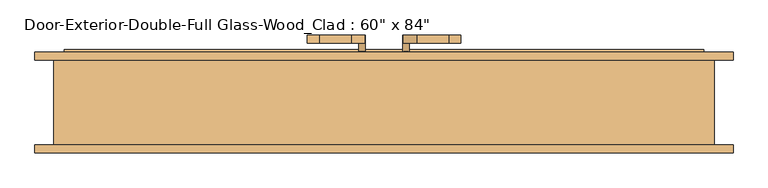
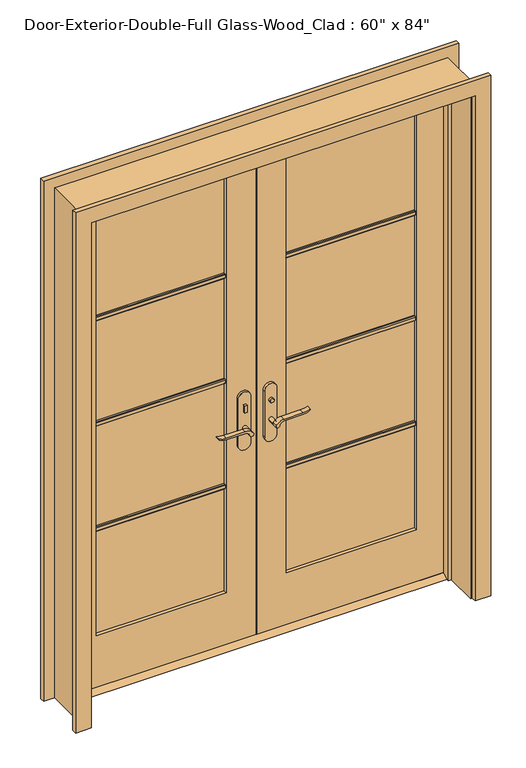
"""IFC4 building model written with IfcOpenShell, lengths in millimetres: door geometry."""

from ifc_helpers import new_model, si_unit, point, frame, frame_2d, origin, place, context, project, spatial, polyline, circle_curve, trimmed, segment, composite_curve, outline, extrude, faceted_brep, source, transform, mapped, element, save


def door_34824ff4(model_context):
    return source(origin(), model_context, "Body", "SolidModel", [
        extrude(outline(polyline([(63.5, 12.7), (98.425, 12.7), (123.825, 0.0), (38.1, 0.0), (63.5, 12.7)])), frame((-762.0, 0.0, 0.0), z_axis=(1.0, 0.0, 0.0), x_axis=(0.0, 1.0, 0.0)), (0.0, 0.0, 1.0), 1524.0),
        extrude(outline(polyline([(-47.4019111, 43.5), (-57.4019111, 43.5), (-57.4019111, 53.5), (-47.4019111, 53.5), (-47.4019111, 43.5)])), frame((0.0, 0.0, 981.9), z_axis=(0.0, 0.0, 1.0), x_axis=(1.0, 0.0, 0.0)), (0.0, 0.0, 1.0), 30.0),
        extrude(outline(composite_curve([segment(trimmed(circle_curve(frame_2d((996.9, -52.4019111)), 8.0), [point((996.9, -60.4019111))], [point((996.9, -44.4019111))], False, "CARTESIAN"), True, "CONTINUOUS"), segment(trimmed(circle_curve(frame_2d((996.9, -52.4019111)), 8.0), [point((996.9, -44.4019111))], [point((996.9, -60.4019111))], False, "CARTESIAN"), True, "CONTINUOUS")], self_intersect=False)), frame((0.0, 108.425, 0.0), z_axis=(0.0, 1.0, 0.0), x_axis=(0.0, 0.0, 1.0)), (0.0, 0.0, 1.0), 10.0),
        extrude(outline(composite_curve([segment(trimmed(circle_curve(frame_2d((897.1555521, -76.0694241)), 37.2832219), [point((919.0523287, -45.8937749))], [point((934.4, -77.7693445))], False, "CARTESIAN"), True, "CONTINUOUS"), segment(polyline([(934.4, -77.7693445), (934.4, -154.045502)]), True, "CONTINUOUS"), segment(trimmed(circle_curve(frame_2d((1017.6850638, -153.9791202)), 83.2850902), [point((934.4, -154.045502))], [point((939.4, -182.4019111))], True, "CARTESIAN"), True, "CONTINUOUS"), segment(polyline([(939.4, -182.4019111), (936.6135558, -182.4019111)]), True, "CONTINUOUS"), segment(trimmed(circle_curve(frame_2d((986.6709207, -150.4622499)), 59.3791355), [point((936.6135558, -182.4019111))], [point((927.4, -154.045502))], False, "CARTESIAN"), True, "CONTINUOUS"), segment(polyline([(927.4, -154.045502), (927.4, -77.7881013)]), True, "CONTINUOUS"), segment(trimmed(circle_curve(frame_2d((909.2738613, -77.7881013)), 18.1261387), [point((927.4, -77.7881013))], [point((914.4, -60.4019111))], True, "CARTESIAN"), True, "CONTINUOUS"), segment(trimmed(circle_curve(frame_2d((914.4, -52.4019111)), 8.0), [point((914.4, -60.4019111))], [point((919.0523287, -45.8937749))], False, "CARTESIAN"), True, "CONTINUOUS")], self_intersect=False)), frame((0.0, 3.5, 0.0), z_axis=(0.0, 1.0, 0.0), x_axis=(0.0, 0.0, 1.0)), (0.0, 0.0, 1.0), 20.0),
        extrude(outline(composite_curve([segment(trimmed(circle_curve(frame_2d((914.4, -52.4019111)), 8.0), [point((914.3999903, -60.4019111))], [point((919.0523287, -45.8937749))], False, "CARTESIAN"), True, "CONTINUOUS"), segment(trimmed(circle_curve(frame_2d((897.1555521, -76.0694241)), 37.2832219), [point((919.0523287, -45.8937749))], [point((934.4, -77.7693445))], False, "CARTESIAN"), True, "CONTINUOUS"), segment(polyline([(934.4, -77.7693445), (934.4, -154.045502)]), True, "CONTINUOUS"), segment(trimmed(circle_curve(frame_2d((1017.6850638, -153.9791202)), 83.2850902), [point((934.4, -154.045502))], [point((939.4, -182.4019111))], True, "CARTESIAN"), True, "CONTINUOUS"), segment(polyline([(939.4, -182.4019111), (936.6135558, -182.4019111)]), True, "CONTINUOUS"), segment(trimmed(circle_curve(frame_2d((986.6709207, -150.4622499)), 59.3791355), [point((936.6135558, -182.4019111))], [point((927.4, -154.045502))], False, "CARTESIAN"), True, "CONTINUOUS"), segment(polyline([(927.4, -154.045502), (927.4, -77.788099)]), True, "CONTINUOUS"), segment(trimmed(circle_curve(frame_2d((909.2738682, -77.788099)), 18.1261318), [point((927.4, -77.788099))], [point((914.3999903, -60.4019111))], True, "CARTESIAN"), True, "CONTINUOUS")], self_intersect=False)), frame((0.0, 138.425, 0.0), z_axis=(0.0, 1.0, 0.0), x_axis=(0.0, 0.0, 1.0)), (0.0, 0.0, 1.0), 20.0),
        extrude(outline(composite_curve([segment(trimmed(circle_curve(frame_2d((914.4, -52.4019111)), 8.0), [point((914.4, -60.4019111))], [point((914.4, -44.4019111))], False, "CARTESIAN"), True, "CONTINUOUS"), segment(trimmed(circle_curve(frame_2d((914.4, -52.4019111)), 8.0), [point((914.4, -44.4019111))], [point((914.4, -60.4019111))], False, "CARTESIAN"), True, "CONTINUOUS")], self_intersect=False)), frame((0.0, 23.5, 0.0), z_axis=(0.0, 1.0, 0.0), x_axis=(0.0, 0.0, 1.0)), (0.0, 0.0, 1.0), 30.0),
        extrude(outline(composite_curve([segment(trimmed(circle_curve(frame_2d((914.4, -52.4019111)), 8.0), [point((914.4, -60.4019111))], [point((914.4, -44.4019111))], False, "CARTESIAN"), True, "CONTINUOUS"), segment(trimmed(circle_curve(frame_2d((914.4, -52.4019111)), 8.0), [point((914.4, -44.4019111))], [point((914.4, -60.4019111))], False, "CARTESIAN"), True, "CONTINUOUS")], self_intersect=False)), frame((0.0, 108.425, 0.0), z_axis=(0.0, 1.0, 0.0), x_axis=(0.0, 0.0, 1.0)), (0.0, 0.0, 1.0), 30.0),
        extrude(outline(composite_curve([segment(polyline([(844.4, -27.4019111), (1039.4, -27.4019111)]), True, "CONTINUOUS"), segment(trimmed(circle_curve(frame_2d((1039.4, -52.4019111)), 25.0), [point((1039.4, -27.4019111))], [point((1039.4, -77.4019111))], False, "CARTESIAN"), True, "CONTINUOUS"), segment(polyline([(1039.4, -77.4019111), (844.4, -77.4019111)]), True, "CONTINUOUS"), segment(trimmed(circle_curve(frame_2d((844.4, -52.4019111)), 25.0), [point((844.4, -77.4019111))], [point((844.4, -27.4019111))], False, "CARTESIAN"), True, "CONTINUOUS")], self_intersect=False)), frame((0.0, 53.5, 0.0), z_axis=(0.0, 1.0, 0.0), x_axis=(0.0, 0.0, 1.0)), (0.0, 0.0, 1.0), 10.0),
        extrude(outline(composite_curve([segment(polyline([(844.4, -27.4019111), (1039.4, -27.4019111)]), True, "CONTINUOUS"), segment(trimmed(circle_curve(frame_2d((1039.4, -52.4019111)), 25.0), [point((1039.4, -27.4019111))], [point((1039.4, -77.4019111))], False, "CARTESIAN"), True, "CONTINUOUS"), segment(polyline([(1039.4, -77.4019111), (844.4, -77.4019111)]), True, "CONTINUOUS"), segment(trimmed(circle_curve(frame_2d((844.4, -52.4019111)), 25.0), [point((844.4, -77.4019111))], [point((844.4, -27.4019111))], False, "CARTESIAN"), True, "CONTINUOUS")], self_intersect=False)), frame((0.0, 98.425, 0.0), z_axis=(0.0, 1.0, 0.0), x_axis=(0.0, 0.0, 1.0)), (0.0, 0.0, 1.0), 10.0),
        extrude(outline(polyline([(47.3875, 118.425), (57.3875, 118.425), (57.3875, 108.425), (47.3875, 108.425), (47.3875, 118.425)])), frame((0.0, 0.0, 981.9), z_axis=(0.0, 0.0, 1.0), x_axis=(1.0, 0.0, 0.0)), (0.0, 0.0, 1.0), 30.0),
        extrude(outline(composite_curve([segment(trimmed(circle_curve(frame_2d((996.9, 52.3875)), 8.0), [point((996.9, 60.3875))], [point((996.9, 44.3875))], False, "CARTESIAN"), True, "CONTINUOUS"), segment(trimmed(circle_curve(frame_2d((996.9, 52.3875)), 8.0), [point((996.9, 44.3875))], [point((996.9, 60.3875))], False, "CARTESIAN"), True, "CONTINUOUS")], self_intersect=False)), frame((0.0, 43.5, 0.0), z_axis=(0.0, 1.0, 0.0), x_axis=(0.0, 0.0, 1.0)), (0.0, 0.0, 1.0), 10.0),
        extrude(outline(composite_curve([segment(trimmed(circle_curve(frame_2d((914.4, 52.3875)), 8.0), [point((919.0523287, 45.8793637))], [point((914.4, 60.3875))], False, "CARTESIAN"), True, "CONTINUOUS"), segment(trimmed(circle_curve(frame_2d((909.2738613, 77.7736901)), 18.1261387), [point((914.4, 60.3875))], [point((927.4, 77.7736901))], True, "CARTESIAN"), True, "CONTINUOUS"), segment(polyline([(927.4, 77.7736901), (927.4, 154.0310909)]), True, "CONTINUOUS"), segment(trimmed(circle_curve(frame_2d((986.6709207, 150.4478388)), 59.3791355), [point((927.4, 154.0310909))], [point((936.6135558, 182.3875))], False, "CARTESIAN"), True, "CONTINUOUS"), segment(polyline([(936.6135558, 182.3875), (939.4, 182.3875)]), True, "CONTINUOUS"), segment(trimmed(circle_curve(frame_2d((1017.6850638, 153.9647091)), 83.2850902), [point((939.4, 182.3875))], [point((934.4, 154.0310909))], True, "CARTESIAN"), True, "CONTINUOUS"), segment(polyline([(934.4, 154.0310909), (934.4, 77.7549333)]), True, "CONTINUOUS"), segment(trimmed(circle_curve(frame_2d((897.1555521, 76.0550129)), 37.2832219), [point((934.4, 77.7549333))], [point((919.0523287, 45.8793637))], False, "CARTESIAN"), True, "CONTINUOUS")], self_intersect=False)), frame((0.0, 138.425, 0.0), z_axis=(0.0, 1.0, 0.0), x_axis=(0.0, 0.0, 1.0)), (0.0, 0.0, 1.0), 20.0),
        extrude(outline(composite_curve([segment(trimmed(circle_curve(frame_2d((909.2738682, 77.7736878)), 18.1261318), [point((914.3999903, 60.3875))], [point((927.4, 77.7736878))], True, "CARTESIAN"), True, "CONTINUOUS"), segment(polyline([(927.4, 77.7736878), (927.4, 154.0310909)]), True, "CONTINUOUS"), segment(trimmed(circle_curve(frame_2d((986.6709207, 150.4478388)), 59.3791355), [point((927.4, 154.0310909))], [point((936.6135558, 182.3875))], False, "CARTESIAN"), True, "CONTINUOUS"), segment(polyline([(936.6135558, 182.3875), (939.4, 182.3875)]), True, "CONTINUOUS"), segment(trimmed(circle_curve(frame_2d((1017.6850638, 153.9647091)), 83.2850902), [point((939.4, 182.3875))], [point((934.4, 154.0310909))], True, "CARTESIAN"), True, "CONTINUOUS"), segment(polyline([(934.4, 154.0310909), (934.4, 77.7549333)]), True, "CONTINUOUS"), segment(trimmed(circle_curve(frame_2d((897.1555521, 76.0550129)), 37.2832219), [point((934.4, 77.7549333))], [point((919.0523287, 45.8793637))], False, "CARTESIAN"), True, "CONTINUOUS"), segment(trimmed(circle_curve(frame_2d((914.4, 52.3875)), 8.0), [point((919.0523287, 45.8793637))], [point((914.3999903, 60.3875))], False, "CARTESIAN"), True, "CONTINUOUS")], self_intersect=False)), frame((0.0, 3.5, 0.0), z_axis=(0.0, 1.0, 0.0), x_axis=(0.0, 0.0, 1.0)), (0.0, 0.0, 1.0), 20.0),
        extrude(outline(composite_curve([segment(trimmed(circle_curve(frame_2d((914.4, 52.3875)), 8.0), [point((914.4, 60.3875))], [point((914.4, 44.3875))], False, "CARTESIAN"), True, "CONTINUOUS"), segment(trimmed(circle_curve(frame_2d((914.4, 52.3875)), 8.0), [point((914.4, 44.3875))], [point((914.4, 60.3875))], False, "CARTESIAN"), True, "CONTINUOUS")], self_intersect=False)), frame((0.0, 108.425, 0.0), z_axis=(0.0, 1.0, 0.0), x_axis=(0.0, 0.0, 1.0)), (0.0, 0.0, 1.0), 30.0),
        extrude(outline(composite_curve([segment(trimmed(circle_curve(frame_2d((914.4, 52.3875)), 8.0), [point((914.4, 60.3875))], [point((914.4, 44.3875))], False, "CARTESIAN"), True, "CONTINUOUS"), segment(trimmed(circle_curve(frame_2d((914.4, 52.3875)), 8.0), [point((914.4, 44.3875))], [point((914.4, 60.3875))], False, "CARTESIAN"), True, "CONTINUOUS")], self_intersect=False)), frame((0.0, 23.5, 0.0), z_axis=(0.0, 1.0, 0.0), x_axis=(0.0, 0.0, 1.0)), (0.0, 0.0, 1.0), 30.0),
        extrude(outline(composite_curve([segment(trimmed(circle_curve(frame_2d((844.4, 52.3875)), 25.0), [point((844.4, 27.3875))], [point((844.4, 77.3875))], False, "CARTESIAN"), True, "CONTINUOUS"), segment(polyline([(844.4, 77.3875), (1039.4, 77.3875)]), True, "CONTINUOUS"), segment(trimmed(circle_curve(frame_2d((1039.4, 52.3875)), 25.0), [point((1039.4, 77.3875))], [point((1039.4, 27.3875))], False, "CARTESIAN"), True, "CONTINUOUS"), segment(polyline([(1039.4, 27.3875), (844.4, 27.3875)]), True, "CONTINUOUS")], self_intersect=False)), frame((0.0, 98.425, 0.0), z_axis=(0.0, 1.0, 0.0), x_axis=(0.0, 0.0, 1.0)), (0.0, 0.0, 1.0), 10.0),
        extrude(outline(composite_curve([segment(trimmed(circle_curve(frame_2d((844.4, 52.3875)), 25.0), [point((844.4, 27.3875))], [point((844.4, 77.3875))], False, "CARTESIAN"), True, "CONTINUOUS"), segment(polyline([(844.4, 77.3875), (1039.4, 77.3875)]), True, "CONTINUOUS"), segment(trimmed(circle_curve(frame_2d((1039.4, 52.3875)), 25.0), [point((1039.4, 77.3875))], [point((1039.4, 27.3875))], False, "CARTESIAN"), True, "CONTINUOUS"), segment(polyline([(1039.4, 27.3875), (844.4, 27.3875)]), True, "CONTINUOUS")], self_intersect=False)), frame((0.0, 53.5, 0.0), z_axis=(0.0, 1.0, 0.0), x_axis=(0.0, 0.0, 1.0)), (0.0, 0.0, 1.0), 10.0),
        extrude(outline(polyline([(77.47, 1578.371875), (77.47, 1559.321875), (71.12, 1559.321875), (67.945, 1562.496875), (67.945, 1575.196875), (71.12, 1578.371875), (77.47, 1578.371875)])), frame((120.65, 0.0, 0.0), z_axis=(1.0, 0.0, 0.0), x_axis=(0.0, 1.0, 0.0)), (0.0, 0.0, 1.0), 520.7),
        extrude(outline(polyline([(77.47, 1132.68125), (77.47, 1113.63125), (71.12, 1113.63125), (67.945, 1116.80625), (67.945, 1129.50625), (71.12, 1132.68125), (77.47, 1132.68125)])), frame((120.65, 0.0, 0.0), z_axis=(1.0, 0.0, 0.0), x_axis=(0.0, 1.0, 0.0)), (0.0, 0.0, 1.0), 520.7),
        extrude(outline(polyline([(77.47, 686.990625), (77.47, 667.940625), (71.12, 667.940625), (67.945, 671.115625), (67.945, 683.815625), (71.12, 686.990625), (77.47, 686.990625)])), frame((120.65, 0.0, 0.0), z_axis=(1.0, 0.0, 0.0), x_axis=(0.0, 1.0, 0.0)), (0.0, 0.0, 1.0), 520.7),
        extrude(outline(polyline([(84.455, 1578.371875), (90.805, 1578.371875), (93.98, 1575.196875), (93.98, 1562.496875), (90.805, 1559.321875), (84.455, 1559.321875), (84.455, 1578.371875)])), frame((-641.35, 0.0, 0.0), z_axis=(1.0, 0.0, 0.0), x_axis=(0.0, 1.0, 0.0)), (0.0, 0.0, 1.0), 520.7),
        extrude(outline(polyline([(84.455, 1132.68125), (90.805, 1132.68125), (93.98, 1129.50625), (93.98, 1116.80625), (90.805, 1113.63125), (84.455, 1113.63125), (84.455, 1132.68125)])), frame((-641.35, 0.0, 0.0), z_axis=(1.0, 0.0, 0.0), x_axis=(0.0, 1.0, 0.0)), (0.0, 0.0, 1.0), 520.7),
        extrude(outline(polyline([(84.455, 686.990625), (90.805, 686.990625), (93.98, 683.815625), (93.98, 671.115625), (90.805, 667.940625), (84.455, 667.940625), (84.455, 686.990625)])), frame((-641.35, 0.0, 0.0), z_axis=(1.0, 0.0, 0.0), x_axis=(0.0, 1.0, 0.0)), (0.0, 0.0, 1.0), 520.7),
        extrude(outline(polyline([(84.455, 1578.371875), (90.805, 1578.371875), (93.98, 1575.196875), (93.98, 1562.496875), (90.805, 1559.321875), (84.455, 1559.321875), (84.455, 1578.371875)])), frame((120.65, 0.0, 0.0), z_axis=(1.0, 0.0, 0.0), x_axis=(0.0, 1.0, 0.0)), (0.0, 0.0, 1.0), 520.7),
        extrude(outline(polyline([(84.455, 1132.68125), (90.805, 1132.68125), (93.98, 1129.50625), (93.98, 1116.80625), (90.805, 1113.63125), (84.455, 1113.63125), (84.455, 1132.68125)])), frame((120.65, 0.0, 0.0), z_axis=(1.0, 0.0, 0.0), x_axis=(0.0, 1.0, 0.0)), (0.0, 0.0, 1.0), 520.7),
        extrude(outline(polyline([(84.455, 686.990625), (90.805, 686.990625), (93.98, 683.815625), (93.98, 671.115625), (90.805, 667.940625), (84.455, 667.940625), (84.455, 686.990625)])), frame((120.65, 0.0, 0.0), z_axis=(1.0, 0.0, 0.0), x_axis=(0.0, 1.0, 0.0)), (0.0, 0.0, 1.0), 520.7),
        extrude(outline(polyline([(77.47, 1578.371875), (77.47, 1559.321875), (71.12, 1559.321875), (67.945, 1562.496875), (67.945, 1575.196875), (71.12, 1578.371875), (77.47, 1578.371875)])), frame((-641.35, 0.0, 0.0), z_axis=(1.0, 0.0, 0.0), x_axis=(0.0, 1.0, 0.0)), (0.0, 0.0, 1.0), 520.7),
        extrude(outline(polyline([(77.47, 1132.68125), (77.47, 1113.63125), (71.12, 1113.63125), (67.945, 1116.80625), (67.945, 1129.50625), (71.12, 1132.68125), (77.47, 1132.68125)])), frame((-641.35, 0.0, 0.0), z_axis=(1.0, 0.0, 0.0), x_axis=(0.0, 1.0, 0.0)), (0.0, 0.0, 1.0), 520.7),
        extrude(outline(polyline([(77.47, 686.990625), (77.47, 667.940625), (71.12, 667.940625), (67.945, 671.115625), (67.945, 683.815625), (71.12, 686.990625), (77.47, 686.990625)])), frame((-641.35, 0.0, 0.0), z_axis=(1.0, 0.0, 0.0), x_axis=(0.0, 1.0, 0.0)), (0.0, 0.0, 1.0), 520.7),
        extrude(outline(polyline([(0.0, 768.35), (0.0, 831.85), (2203.45, 831.85), (2203.45, -831.85), (0.0, -831.85), (0.0, -768.35), (2139.95, -768.35), (2139.95, 768.35), (0.0, 768.35)])), frame((0.0, 98.425, 0.0), z_axis=(0.0, 1.0, 0.0), x_axis=(0.0, 0.0, 1.0)), (0.0, 0.0, 1.0), 19.05),
        extrude(outline(polyline([(0.0, 768.35), (0.0, 831.85), (2203.45, 831.85), (2203.45, -831.85), (0.0, -831.85), (0.0, -768.35), (2139.95, -768.35), (2139.95, 768.35), (0.0, 768.35)])), frame((0.0, -123.825, 0.0), z_axis=(0.0, 1.0, 0.0), x_axis=(0.0, 0.0, 1.0)), (0.0, 0.0, 1.0), 19.05),
        extrude(outline(polyline([(12.7, 762.0), (2133.6, 762.0), (2133.6, 1.5875), (12.7, 1.5875), (12.7, 762.0)]), holes=[polyline([(2014.5375, 120.65), (2014.5375, 641.35), (231.775, 641.35), (231.775, 120.65), (2014.5375, 120.65)])]), frame((0.0, 63.5, 0.0), z_axis=(0.0, 1.0, 0.0), x_axis=(0.0, 0.0, 1.0)), (0.0, 0.0, 1.0), 34.925),
        extrude(outline(polyline([(2133.6, -762.0), (12.7, -762.0), (12.7, -1.6019111), (2133.6, -1.6019111), (2133.6, -762.0)]), holes=[polyline([(231.775, -641.35), (2014.5375, -641.35), (2014.5375, -120.65), (231.775, -120.65), (231.775, -641.35)])]), frame((0.0, 63.5, 0.0), z_axis=(0.0, 1.0, 0.0), x_axis=(0.0, 0.0, 1.0)), (0.0, 0.0, 1.0), 34.925),
        faceted_brep([(787.4, 98.425, 0.0), (787.4, -104.775, 0.0), (762.0, -104.775, 0.0), (762.0, 28.575, 0.0), (749.3, 28.575, 0.0), (749.3, 63.5, 0.0), (762.0, 63.5, 0.0), (762.0, 98.425, 0.0), (787.4, 98.425, 2159.0), (787.4, -104.775, 2159.0), (-787.4, -104.775, 2159.0), (-787.4, -104.775, 0.0), (-762.0, -104.775, 0.0), (-762.0, -104.775, 2133.6), (762.0, -104.775, 2133.6), (762.0, 28.575, 2133.6), (-762.0, 28.575, 2133.6), (-762.0, 28.575, 0.0), (-749.3, 28.575, 0.0), (-749.3, 28.575, 2120.9), (749.3, 28.575, 2120.9), (749.3, 63.5, 2120.9), (1.5875, 63.5, 2120.9), (-1.6019111, 63.5, 2120.9), (-749.3, 63.5, 2120.9), (-749.3, 63.5, 0.0), (-762.0, 63.5, 0.0), (-762.0, 63.5, 2133.6), (-1.6019111, 63.5, 2133.6), (1.5875, 63.5, 2133.6), (762.0, 63.5, 2133.6), (762.0, 98.425, 2133.6), (1.5875, 98.425, 2133.6), (-1.6019111, 98.425, 2133.6), (-762.0, 98.425, 2133.6), (-762.0, 98.425, 0.0), (-787.4, 98.425, 0.0), (-787.4, 98.425, 2159.0)], [[[0, 1, 2, 3, 4, 5, 6, 7]], [[1, 0, 8, 9]], [[2, 1, 9, 10, 11, 12, 13, 14]], [[3, 2, 14, 15]], [[4, 3, 15, 16, 17, 18, 19, 20]], [[5, 4, 20, 21]], [[6, 5, 21, 22, 23, 24, 25, 26, 27, 28, 29, 30]], [[7, 6, 30, 31]], [[0, 7, 31, 32, 33, 34, 35, 36, 37, 8]], [[9, 8, 37, 10]], [[14, 13, 16, 15]], [[20, 19, 24, 23, 22, 21]], [[31, 30, 29, 28, 27, 34, 33, 32]], [[12, 11, 36, 35, 26, 25, 18, 17]], [[11, 10, 37, 36]], [[13, 12, 17, 16]], [[19, 18, 25, 24]], [[27, 26, 35, 34]]]),
        extrude(outline(polyline([(641.35, 77.47), (120.65, 77.47), (120.65, 84.455), (641.35, 84.455), (641.35, 77.47)])), frame((0.0, 0.0, 231.775), z_axis=(0.0, 0.0, 1.0), x_axis=(1.0, 0.0, 0.0)), (0.0, 0.0, 1.0), 1782.7625),
        extrude(outline(polyline([(-120.65, 77.47), (-641.35, 77.47), (-641.35, 84.455), (-120.65, 84.455), (-120.65, 77.47)])), frame((0.0, 0.0, 231.775), z_axis=(0.0, 0.0, 1.0), x_axis=(1.0, 0.0, 0.0)), (0.0, 0.0, 1.0), 1782.7625),
    ])


if __name__ == "__main__":
    model = new_model("IFC4")
    model_context = context("Model", 3, world=origin())
    ifc_project = project(units=[si_unit("LENGTHUNIT", "METRE", prefix="MILLI")], contexts=[model_context])
    site = spatial("IfcSite", under=ifc_project)
    building = spatial("IfcBuilding", under=site)
    placement = place(None, origin())
    door_shape = door_34824ff4(model_context)
    element("IfcDoor", 1, ObjectType="Door-Exterior-Double-Full Glass-Wood_Clad : 60\" x 84\"", at=placement, inside=building, context=model_context, shape_type="MappedRepresentation", body=[
        mapped(door_shape, transform((0.0, 0.0, 0.0), x_axis=(1.0, 0.0, 0.0), y_axis=(0.0, 1.0, 0.0), z_axis=(0.0, 0.0, 1.0))),
    ])
    save(model, "model.ifc")

# Revit data of these elements
# Type "Door-Exterior-Double-Full Glass-Wood_Clad : 60\" x 84\""
#   Type Mark = "8"
#   Assembly Code = "B2030100"
#   Analytic Construction = "French door, wood frame with double glass"
#   Top Rail = 0' - 4 11/16"
#   Threshold Offset [instance default] = 0' - 0 1/2"
#   Thickness = 0' - 1 3/8"
#   Thermal Resistance (R) = 0.337392 (m²·K)/W
#   Swing Angle [instance default] = 90.00°
#   Stiles = 0' - 4 3/4"
#   Rough Width = 5' - 2"
#   Rough Height = 7' - 1"
#   Panel Width = 2' - 6"
#   Door Offset [instance default] = 0' - 0"
#   Height = 7' - 0"
#   Width = 5' - 0"
#   Heat Transfer Coefficient (U) = 2.96405 W/(m²·K)
#   Bottom Rail = 0' - 9 1/8"
#   Exterior Trim [instance default] = yes
#   Threshold [instance default] = yes
#   Show Grill [instance default] = yes
#   Function = 1
#   Trim Material = Cherry
#   Threshold Material = Cherry
#   Panel Material = Cherry
#   Glazing = Glass
#   Frame Material = Cherry
#   Door Handle Material = Aluminum
#   Visual Light Transmittance = 0
#   Solar Heat Gain Coefficient = 0
#   Wall Closure = (empty or 0)
#   Construction Type = (empty or 0)
# Element 1 (IfcDoor, "Door-Exterior-Double-Full Glass-Wood_Clad : 60\" x 84\"")
#   Materials on its faces: "Cherry", "Aluminum", "Glass"
# Materials
#   "Cherry": class "Wood", colour RGB 226 177 128, transparency 0, Description = "Prunus Serotina", Cost = 0
#   "Glass": class "Glass", colour RGB 0 128 192, transparency 0.75, Description = "Soda Lime Glass", Cost = 0
#   "Aluminum": class "Metal", colour RGB 247 247 247, transparency 0, Description = "Aluminum 6061", Cost = 0
